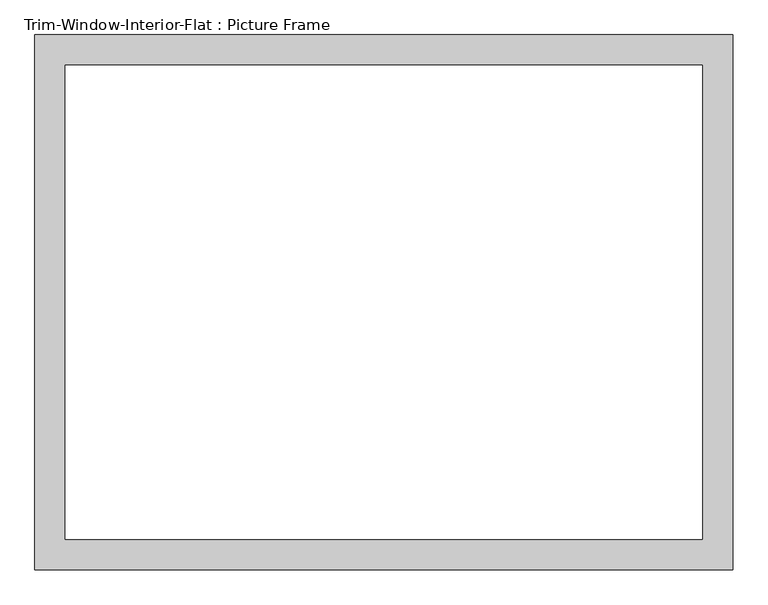
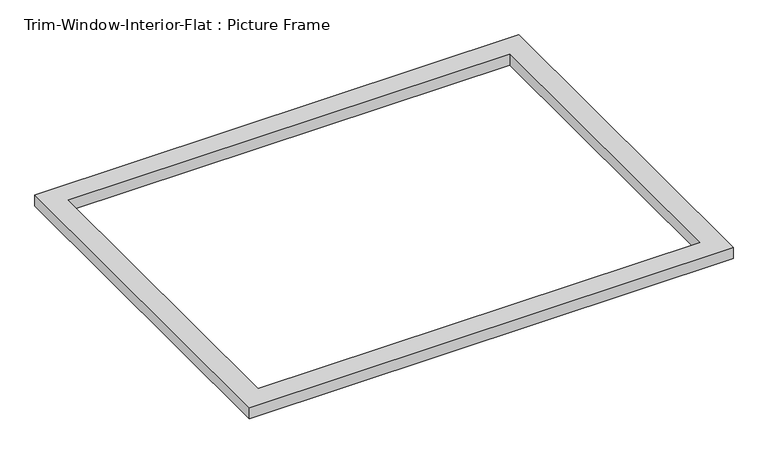
"""IFC4 building model written with IfcOpenShell, lengths in millimetres: proxy geometry, Trim-Window-Interior-Flat : Picture Frame."""

from ifc_helpers import new_model, si_unit, origin, origin_with_axes, place, context, project, spatial, polyline, outline, extrude, source, transform, mapped, element, save


def trim_window_interior_flat_picture_frame_5593adf3(model_context):
    return source(origin(), model_context, "Body", "SweptSolid", [
        extrude(outline(polyline([(654.05, -44.45), (-654.05, -44.45), (-654.05, 958.85), (654.05, 958.85), (654.05, -44.45)]), holes=[polyline([(596.9, 12.7), (596.9, 901.7), (-596.9, 901.7), (-596.9, 12.7), (596.9, 12.7)])]), origin_with_axes(), (0.0, 0.0, 1.0), 31.75),
    ])


if __name__ == "__main__":
    model = new_model("IFC4")
    model_context = context("Model", 3, world=origin())
    ifc_project = project(units=[si_unit("LENGTHUNIT", "METRE", prefix="MILLI")], contexts=[model_context])
    site = spatial("IfcSite", under=ifc_project)
    building = spatial("IfcBuilding", under=site)
    placement = place(None, origin())
    trim_window_interior_flat_picture_frame_shape = trim_window_interior_flat_picture_frame_5593adf3(model_context)
    element("IfcBuildingElementProxy", 1, Name="Trim-Window-Interior-Flat : Picture Frame", ObjectType="Trim-Window-Interior-Flat : Picture Frame", at=placement, inside=building, context=model_context, shape_type="MappedRepresentation", body=[
        mapped(trim_window_interior_flat_picture_frame_shape, transform((0.0, 0.0, 0.0), x_axis=(1.0, 0.0, 0.0), y_axis=(0.0, 1.0, 0.0), z_axis=(0.0, 0.0, 1.0))),
    ])
    save(model, "model.ifc")

# Revit data of these elements
# Type "Trim-Window-Interior-Flat : Picture Frame"
#   Trim Thickness_Picture Frame = 0' - 1 1/4"
#   Trim Width = 0' - 2 1/4"
#   Trim Thickness_with Sill = 0' - 0 3/4"
#   Sill Thickness = 0' - 1 1/4"
#   Opening Width [instance default] = 2' - 0"
#   Opening Height [instance default] = 3' - 0"
#   Default Elevation = 4' - 0"
#   Sill = no
#   Picture Frame = yes
#   Trim Material [instance default] = none
# Element 1 (IfcBuildingElementProxy, "Trim-Window-Interior-Flat : Picture Frame")
#   Opening Width = 4' - 0"
#   Trim Material = Wood - Stained
#   Materials on its faces: "Wood - Stained"
# Materials
#   "Wood - Stained": class "Wood", colour RGB 224 178 126, transparency 0, Cost = 0
